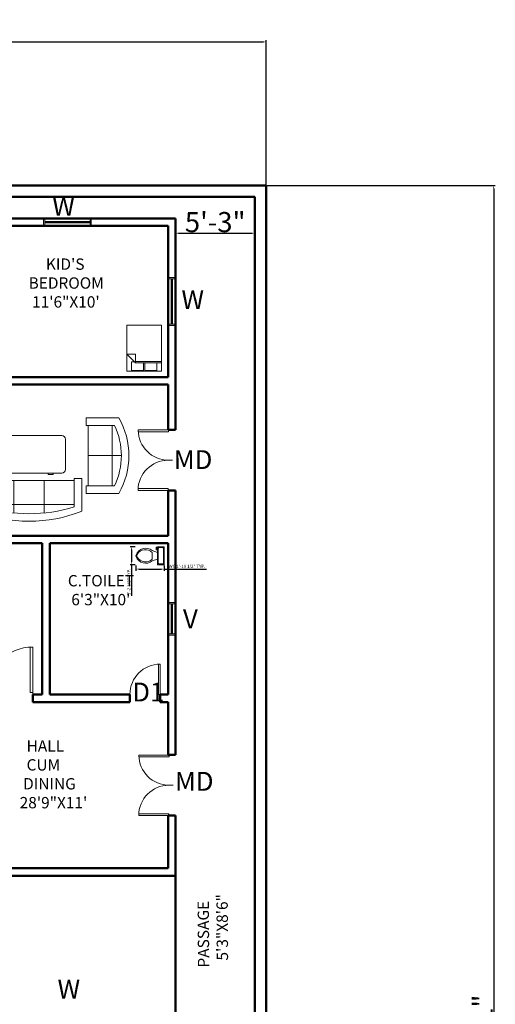
# Model space of a CAD drawing. Units: inches. Extents: x -7040 to -4088, y 6092 to 7645.
# Tile 7 of 11: x -6599 to -6221, y 6864 to 7645. Entities that reach past the tile are written whole.
import ezdxf

# ---------------------------------------------------------------- set-up
doc = ezdxf.new("R2010")
doc.units = ezdxf.units.IN
for name, color, linetype, lineweight in [('A-ANNO-DIMS', 2, 'Continuous', 18), ('A-ANNO-TEXT', 7, 'Continuous', 25), ('A-AREA-IDEN', 3, 'Continuous', 25), ('A-DOOR', 3, 'Continuous', 18), ('A-FLOR-FIXT', 9, 'Continuous', 13), ('A-FURN', 8, 'Continuous', 13), ('A-GLAZ', 4, 'Continuous', 18), ('A-WALL', 7, 'Continuous', 50)]:
    doc.layers.add(name, color=color, linetype=linetype, lineweight=lineweight)
doc.styles.get("Standard").update_dxf_attribs({"font": 'arial.ttf'})
doc.dimstyles.new('ISO-25', dxfattribs={"dimtxt": 2.5, "dimasz": 2.5, "dimexe": 1.25, "dimexo": 0.625, "dimtad": 1, "dimdec": 0, "dimlunit": 3, "dimtxsty": 'Standard', "dimcen": 2.5, "dimadec": 0, "dimazin": 0, "dimtfac": 1, "dimtdec": 0, "dimtmove": 0, "dimatfit": 3, "dimfxl": 1, "dimarcsym": 0})

# ---------------------------------------------------------------- blocks, each defined once
blk = doc.blocks.new('*U8')
for p, q in [((0, 0), (0, -100)), ((750, 0), (750, -100))]:
    blk.add_line(p, q)
blk.add_lwpolyline([(0, 0), (0, 750), (43.75, 750), (43.75, 0)], close=True)
blk.add_arc((0, 0), 750, 0, 90)
blk = doc.blocks.new('Bed - Queen')
for p, q in [((0, -80.00003), (0, 0)), ((0, 0), (59.99999, 0)), ((59.99999, 0), (59.99999, -80.00003)), ((0, -14.4), (44.8, -14.4)), ((44.8, -16.8), (0, -16.8)), ((7.99999, -1.2), (28.79998, -1.2)), ((7.99999, -14.4), (7.99999, -1.2)), ((28.79998, -1.2), (28.79998, -14.4)), ((31.19999, -1.2), (51.99999, -1.2)), ((31.19999, -14.4), (31.19999, -1.2)), ((59.99999, -29.6), (44.8, -14.4)), ((44.8, -14.4), (44.8, -29.6)), ((51.99999, -16.4), (46.79936, -16.4)), ((51.99999, -1.2), (51.99999, -16.4)), ((44.8, -29.6), (59.99999, -29.6)), ((59.99999, -80.00003), (0, -80.00003))]:
    blk.add_line(p, q)
blk = doc.blocks.new('Toilet - top')
for p, q in [((-10, -8.5), (-8, -8.5)), ((-10, -9.5), (-10, -8.5)), ((-7, -9.5), (-10, -9.5)), ((-8, -8.5), (-8, -8)), ((-7, -8), (-7, -9.5)), ((-4, -8), (-6, -14)), ((4, -8), (6, -14)), ((9.5, -6), (9.5, -2)), ((4, -14), (-4, -14))]:
    blk.add_line(p, q)
blk.add_lwpolyline([(10.5, -8), (10.5, 0), (-10.5, 0), (-10.5, -8)], close=True)
for points in [[(-9.5, -2), (-9.5, -6)], [(8.5, -1), (-8.5, -1)], [(-8.5, -7), (8.5, -7)]]:
    blk.add_lwpolyline(points)
for centre, radius, start, end in [((-8.6, -1.9), 0.884, 81.8699, 188.1301), ((-8.6, -6.1), 0.884, 171.8699, 278.1301), ((8.6, -1.9), 0.884, 351.8699, 98.1301), ((8.6, -6.1), 0.884, 261.8699, 8.1301), ((3.5, -21.6), 12.2, 141.4691, 247.9714), ((4.2, -21.8), 11.3, 136.3677, 238.9468), ((-3.5, -21.6), 12.2, 292.0284, 38.5307), ((-4.2, -21.8), 11.3, 301.053, 43.6321), ((0, -27.9), 4, 245.7318, 294.2682), ((0, -29), 4, 254.8605, 285.1395)]:
    blk.add_arc(centre, radius, start, end)
blk = doc.blocks.new('Desk - 30 x 60 in.')
for p, q in [((-26.999995, 0), (26.999995, 0)), ((-29.999995, -27), (-29.999995, -3)), ((29.999995, -3), (29.999995, -27)), ((26.999995, -30), (-26.999995, -30)), ((-20.000005, -30), (-20.000005, -31)), ((-20.000005, -31), (-16.000005, -31)), ((-16.000005, -31), (-16.000005, -30)), ((15.999995, -31), (15.999995, -30)), ((19.999995, -31), (15.999995, -31)), ((19.999995, -30), (19.999995, -31))]:
    blk.add_line(p, q)
for centre, start, end in [((-26.499995, -3.5), 98.1301, 171.8699), ((26.499995, -3.5), 8.130102, 81.8699), ((-26.499995, -26.5), 188.1301, 261.8699), ((26.499995, -26.5), 278.1301, 351.8699)]:
    blk.add_arc(centre, 3.535534, start, end)
blk = doc.blocks.new('Sofa - Roundback 7 ft.')
for p, q in [((-12.00002, -32.4421), (-12.00003, -6.5971)), ((11.99997, -32.4421), (11.99998, -6.5971)), ((-36.000027, -34), (-36.000027, -11.4696)), ((-35.999844, -13.3819), (35.9998, -13.3819)), ((35.99998, -34), (35.99998, -11.4696)), ((-36.000027, -32.4421), (35.99998, -32.4421))]:
    blk.add_line(p, q)
for points in [[(-36.000027, -34), (-42.000027, -34), (-42.000027, -8)], [(41.99998, -8), (41.99998, -34), (35.99998, -34)]]:
    blk.add_lwpolyline(points)
for centre, radius, start, end in [((0, -114.25), 114.25, 68.43141, 111.5686), ((-0.00001, -127.1968), 121.1968, 72.72033, 107.2797)]:
    blk.add_arc(centre, radius, start, end)
blk = doc.blocks.new('Sofa - Roundback Loveseat 5 ft.')
for p, q in [((0, -32.44198), (0, -5.99998)), ((-24, -33.99998), (-24, -11.46958)), ((-23.9998, -13.38178), (23.99986, -13.38178)), ((24.00004, -33.99998), (24.00004, -11.46958)), ((-24, -32.44198), (24.00004, -32.44198))]:
    blk.add_line(p, q)
for points in [[(-24, -33.99998), (-30, -33.99998), (-30, -7.99998)], [(30.00004, -7.99998), (30.00004, -33.99998), (24.00004, -33.99998)]]:
    blk.add_lwpolyline(points)
for centre, radius, start, end in [((0, -60.24998), 60.24998, 60.13715, 119.8628), ((0, -61.38438), 55.38444, 64.32083, 115.6792)]:
    blk.add_arc(centre, radius, start, end)
blk = doc.blocks.new('*D90')
at = {"layer": 'A-ANNO-DIMS', "color": 0, "lineweight": -2, "transparency": 16777216}
for p, q in [((-6475.03, 7487.13), (-6475.03, 7474.72)), ((-6412.03, 7487.13), (-6412.03, 7474.72)), ((-6472.53, 7475.97), (-6414.53, 7475.97))]:
    blk.add_line(p, q, dxfattribs=at)
at = {"layer": 'A-ANNO-DIMS', "color": 0, "transparency": 16777216}
for points in [[(-6472.53, 7476.38), (-6472.53, 7475.55), (-6475.03, 7475.97)], [(-6414.53, 7476.38), (-6414.53, 7475.55), (-6412.03, 7475.97)]]:
    blk.add_solid(points, dxfattribs=at)
at = {"layer": 'Defpoints', "color": 0, "transparency": 16777216}
for p in [(-6475.03, 7487.76), (-6412.03, 7487.76), (-6412.03, 7475.97)]:
    blk.add_point(p, dxfattribs=at)
at = {"layer": 'A-ANNO-DIMS', "color": 0, "transparency": 16777216, "insert": (-6443.53, 7484.77), "char_height": 2.5, "attachment_point": 5}
blk.add_mtext('{\\H6.4x;5\'-3"}', dxfattribs=at)
blk = doc.blocks.new('*D92')
at = {"layer": 'A-ANNO-DIMS', "color": 0, "lineweight": -2, "transparency": 16777216}
for p, q in [((-7003.03, 7514.38), (-7003.03, 7629.1)), ((-7000.53, 7627.85), (-6405.53, 7627.85)), ((-6403.03, 7514.38), (-6403.03, 7629.1))]:
    blk.add_line(p, q, dxfattribs=at)
at = {"layer": 'A-ANNO-DIMS', "color": 0, "transparency": 16777216}
for points in [[(-7000.53, 7628.27), (-7000.53, 7627.43), (-7003.03, 7627.85)], [(-6405.53, 7628.27), (-6405.53, 7627.43), (-6403.03, 7627.85)]]:
    blk.add_solid(points, dxfattribs=at)
at = {"layer": 'Defpoints', "color": 0, "transparency": 16777216}
for p in [(-6403.03, 7627.85), (-7003.03, 7513.76), (-6403.03, 7513.76)]:
    blk.add_point(p, dxfattribs=at)
at = {"layer": 'A-ANNO-DIMS', "color": 0, "transparency": 16777216, "insert": (-6703.03, 7636.64), "char_height": 2.5, "attachment_point": 5}
blk.add_mtext("{\\H6.4x;50'}", dxfattribs=at)
blk = doc.blocks.new('*D93')
at = {"layer": 'A-ANNO-DIMS', "color": 0, "lineweight": -2, "transparency": 16777216}
for p, q in [((-6402.41, 7513.76), (-6220.88, 7513.76)), ((-6222.13, 7511.26), (-6222.13, 6159.26)), ((-6402.41, 6156.76), (-6220.88, 6156.76))]:
    blk.add_line(p, q, dxfattribs=at)
at = {"layer": 'A-ANNO-DIMS', "color": 0, "transparency": 16777216}
for points in [[(-6222.55, 7511.26), (-6221.71, 7511.26), (-6222.13, 7513.76)], [(-6222.55, 6159.26), (-6221.71, 6159.26), (-6222.13, 6156.76)]]:
    blk.add_solid(points, dxfattribs=at)
at = {"layer": 'Defpoints', "color": 0, "transparency": 16777216}
for p in [(-6403.03, 7513.76), (-6403.03, 6156.76), (-6222.13, 6156.76)]:
    blk.add_point(p, dxfattribs=at)
at = {"layer": 'A-ANNO-DIMS', "color": 0, "transparency": 16777216, "insert": (-6230.93, 6835.26), "char_height": 2.5, "attachment_point": 5, "rotation": 90}
blk.add_mtext('{\\H6.4x;113\'-1"}', dxfattribs=at)
blk = doc.blocks.new('WIN-36')
for p, q in [((0, 6), (0, 0)), ((1, 6), (1, 0)), ((1, 3.5), (37, 3.5)), ((1, 3), (37, 3)), ((1, 2.5), (37, 2.5)), ((37, 6), (37, 0)), ((38, 6), (38, 0))]:
    blk.add_line(p, q)
blk = doc.blocks.new('WIN-24')
for p, q in [((0, 6), (0, 0)), ((1, 6), (1, 0)), ((1, 3.5), (25, 3.5)), ((1, 3), (25, 3)), ((1, 2.5), (25, 2.5)), ((25, 6), (25, 0)), ((26, 6), (26, 0))]:
    blk.add_line(p, q)
blk = doc.blocks.new('*D128')
at = {"layer": 'A-ANNO-DIMS', "color": 0, "lineweight": -2, "transparency": 16777216}
for p, q in [((-6506.58, 7212.04), (-6506.58, 7208.03)), ((-6504.08, 7209.28), (-6486.48, 7209.28)), ((-6483.98, 7212.04), (-6483.98, 7208.03)), ((-6483.98, 7209.28), (-6450.33, 7209.28))]:
    blk.add_line(p, q, dxfattribs=at)
at = {"layer": 'A-ANNO-DIMS', "color": 0, "transparency": 16777216}
for points in [[(-6504.08, 7209.7), (-6504.08, 7208.86), (-6506.58, 7209.28)], [(-6486.48, 7209.7), (-6486.48, 7208.86), (-6483.98, 7209.28)]]:
    blk.add_solid(points, dxfattribs=at)
at = {"layer": 'Defpoints', "color": 0, "transparency": 16777216}
for p in [(-6506.58, 7212.67), (-6483.98, 7212.67), (-6483.98, 7209.28)]:
    blk.add_point(p, dxfattribs=at)
at = {"layer": 'A-ANNO-DIMS', "color": 0, "transparency": 16777216, "insert": (-6465.91, 7211.2), "char_height": 2.5, "attachment_point": 5}
blk.add_mtext('WC 1\'-10 1/2" TYP.', dxfattribs=at)
blk = doc.blocks.new('*D129')
at = {"layer": 'A-ANNO-DIMS', "color": 0, "lineweight": -2, "transparency": 16777216}
for p, q in [((-6507.2, 7227.03), (-6511.22, 7227.03)), ((-6509.97, 7224.53), (-6509.97, 7215.17)), ((-6507.2, 7212.67), (-6511.22, 7212.67)), ((-6509.97, 7212.67), (-6509.97, 7188.09))]:
    blk.add_line(p, q, dxfattribs=at)
at = {"layer": 'A-ANNO-DIMS', "color": 0, "transparency": 16777216}
for points in [[(-6510.38, 7224.53), (-6509.55, 7224.53), (-6509.97, 7227.03)], [(-6510.38, 7215.17), (-6509.55, 7215.17), (-6509.97, 7212.67)]]:
    blk.add_solid(points, dxfattribs=at)
at = {"layer": 'Defpoints', "color": 0, "transparency": 16777216}
for p in [(-6506.58, 7227.03), (-6509.97, 7212.67), (-6506.58, 7212.67)]:
    blk.add_point(p, dxfattribs=at)
at = {"layer": 'A-ANNO-DIMS', "color": 0, "transparency": 16777216, "insert": (-6511.89, 7199.13), "char_height": 2.5, "attachment_point": 5, "rotation": 90}
blk.add_mtext('1\'-2 1/2" TYP.', dxfattribs=at)

msp = doc.modelspace()

# ---------------------------------------------------------------- linework, layer by layer
at = {"layer": 'A-WALL'}
for p, q in [((-7003.03, 7513.76), (-6403.03, 7513.76)), ((-6403.03, 7513.76), (-6403.03, 6156.76)), ((-6994.03, 7504.76), (-6412.03, 7504.76)), ((-6412.03, 7504.76), (-6412.03, 6179.76)), ((-6977.03, 7487.76), (-6475.03, 7487.76)), ((-6641.03, 7481.76), (-6481.03, 7481.76)), ((-6481.03, 7481.76), (-6481.03, 7361.76)), ((-6475.03, 7487.76), (-6475.03, 7319.76)), ((-6641.03, 7361.76), (-6481.03, 7361.76)), ((-6845.03, 7355.76), (-6481.03, 7355.76)), ((-6481.03, 7355.76), (-6481.03, 7319.76)), ((-6481.03, 7319.76), (-6475.03, 7319.76)), ((-6481.03, 7271.76), (-6475.03, 7271.76)), ((-6481.03, 7271.76), (-6481.03, 7235.76)), ((-6475.03, 7271.76), (-6475.03, 7061.76)), ((-6845.03, 7235.76), (-6481.03, 7235.76)), ((-6773.03, 7229.76), (-6581.03, 7229.76)), ((-6581.03, 7109.76), (-6581.03, 7229.76)), ((-6575.03, 7109.76), (-6575.03, 7229.76)), ((-6575.03, 7229.76), (-6481.03, 7229.76)), ((-6481.03, 7229.76), (-6481.03, 7109.76)), ((-6588.57, 7109.76), (-6588.57, 7103.76)), ((-6588.57, 7109.76), (-6581.03, 7109.76)), ((-6575.03, 7109.76), (-6511.28, 7109.76)), ((-6511.28, 7109.76), (-6511.28, 7103.76)), ((-6487.28, 7109.76), (-6487.28, 7103.76)), ((-6487.28, 7109.76), (-6481.03, 7109.76)), ((-6588.57, 7103.76), (-6511.28, 7103.76)), ((-6487.28, 7103.76), (-6481.03, 7103.76)), ((-6481.03, 7103.76), (-6481.03, 7061.76)), ((-6481.03, 7061.76), (-6475.03, 7061.76)), ((-6481.03, 7013.76), (-6475.03, 7013.76)), ((-6481.03, 7013.76), (-6481.03, 6971.76)), ((-6475.03, 7013.76), (-6475.03, 6658.26)), ((-6971.03, 6965.76), (-6475.03, 6965.76)), ((-6845.03, 6971.76), (-6481.03, 6971.76))]:
    msp.add_line(p, q, dxfattribs=at)

# ---------------------------------------------------------------- block references
at = {"layer": 'A-DOOR'}
for p, xscale, yscale, zscale, rotation in [((-6480.69, 7319.76), -0.0319999999999999, 0.0319999999999999, 0.0319999999999999, 90), ((-6480.87, 7271.76), 0.0319965751455487, 0.0319965751455487, 0.0319965751455487, 90.00000000000003), ((-6480.16, 7061.66), -0.0319999999999999, 0.0319999999999999, 0.0319999999999999, 90), ((-6480.34, 7013.65), 0.0319965751455487, 0.0319965751455487, 0.0319965751455487, 90.00000000000003)]:
    msp.add_blockref('*U8', p, dxfattribs=dict(at, xscale=xscale, yscale=yscale, zscale=zscale, rotation=rotation))
for p, xscale, yscale, zscale in [((-6588.57, 7111.39), -0.0480000000000005, 0.0480000000000005, 0.0480000000000005), ((-6487.28, 7109.85), -0.0319999981882539, 0.0319999981882539, 0.0319999981882539)]:
    msp.add_blockref('*U8', p, dxfattribs=dict(at, xscale=xscale, yscale=yscale, zscale=zscale))
at = {"layer": 'A-FLOR-FIXT', "xscale": 0.6837915443005316, "yscale": 0.6837915443005316, "zscale": 0.6837915443005316, "rotation": 270}
msp.add_blockref('Toilet - top', (-6483.98, 7219.85), dxfattribs=at)
at = {"layer": 'A-FURN', "xscale": 0.4580400962997241, "yscale": 0.4580400962997241, "zscale": 0.4580400962997241, "rotation": 180}
msp.add_blockref('Bed - Queen', (-6486.3, 7366.43), dxfattribs=at)
at = {"layer": 'A-FURN'}
for name, p, rotation in [('Sofa - Roundback Loveseat 5 ft.', (-6512.11, 7299.37), 270), ('Sofa - Roundback 7 ft.', (-6591.57, 7247.24), 180)]:
    msp.add_blockref(name, p, dxfattribs=dict(at, rotation=rotation))
msp.add_blockref('Desk - 30 x 60 in.', (-6592.41, 7315.38), dxfattribs=at)
at = {"layer": 'A-GLAZ'}
msp.add_blockref('WIN-36', (-6580.03, 7481.76), dxfattribs=at)
for name, p, rotation in [('WIN-36', (-6475.03, 7402.76), 89.99999999999507), ('WIN-24', (-6481.03, 7182.76), 269.9999999999992)]:
    msp.add_blockref(name, p, dxfattribs=dict(at, rotation=rotation))

# ---------------------------------------------------------------- texts
at = {"layer": 'A-ANNO-TEXT', "char_height": 15, "attachment_point": 1}
for s, insert in [('{W}', (-6573.06, 7504.84)), ('{W}', (-6470.39, 7430.73)), ('{MD}', (-6476.46, 7303.7)), ('{V}', (-6469.14, 7177.29)), ('{D1}', (-6509.46, 7119.17)), ('{MD}', (-6475.55, 7048.27)), ('{W}', (-6568.85, 6883.34))]:
    msp.add_mtext_dynamic_manual_height_columns(s, width=701.5203, gutter_width=12.5, heights=[0], dxfattribs=dict(at, insert=insert))
at = {"layer": 'A-AREA-IDEN', "char_height": 9, "attachment_point": 1}
for s, insert in [('{     KID\'S\\PBEDROOM\\P 11\'6"X10\'}', (-6591.84, 7455.91)), ('{  C.TOILET\\P   6\'3"X10\'}', (-6566.15, 7204.57)), ('{  HALL\\P  CUM\\P DINING\\P28\'9"X11\'}', (-6598.95, 7073.36))]:
    msp.add_mtext_dynamic_manual_height_columns(s, width=930.9751, gutter_width=12.5, heights=[0], dxfattribs=dict(at, insert=insert))
at = {"layer": 'A-AREA-IDEN', "insert": (-6457.21, 6881.89), "char_height": 9, "attachment_point": 1, "rotation": 90.30994}
msp.add_mtext_dynamic_manual_height_columns('{    PASSAGE\\P      5\'3"X8\'6"}', width=930.9751, gutter_width=12.5, heights=[0], dxfattribs=at)

# ---------------------------------------------------------------- dimensions: what is measured, and where the dimension line sits
at = {"layer": 'A-ANNO-DIMS'}
for base, p1, p2, text, override, picture, middle in [((-6403.03, 7627.85), (-7003.03, 7513.76), (-6403.03, 7513.76), '{\\H6.4x;<>}', {"dimclrd": 0, "dimclre": 0, "dimclrt": 0}, '*D92', (-6703.03, 7636.64)), ((-6412.03, 7475.97), (-6475.03, 7487.76), (-6412.03, 7487.76), '{\\H6.4x;<>}', {"dimclrd": 0, "dimclre": 0, "dimclrt": 0}, '*D90', (-6443.53, 7484.77)), ((-6483.98, 7209.28), (-6506.58, 7212.67), (-6483.98, 7212.67), 'WC <> TYP.', {"dimdec": 1, "dimrnd": 0, "dimzin": 1, "dimlunit": 4, "dimfrac": 2}, '*D128', (-6465.91, 7211.2))]:
    dim = msp.add_linear_dim(base=base, p1=p1, p2=p2, text=text, dimstyle='ISO-25', override=override, dxfattribs=at)
    dim.commit()
    dim.dimension.update_dxf_attribs({"geometry": picture, "text_midpoint": middle})
for base, p1, p2, angle, text, override, picture, middle in [((-6222.13, 6156.76), (-6403.03, 7513.76), (-6403.03, 6156.76), 90, '{\\H6.4x;<>}', {"dimclrd": 0, "dimclre": 0, "dimclrt": 0}, '*D93', (-6230.93, 6835.26)), ((-6509.97, 7212.67), (-6506.58, 7227.03), (-6506.58, 7212.67), 270, '<> TYP.', {"dimdec": 1, "dimrnd": 0, "dimzin": 1, "dimlunit": 4, "dimfrac": 2}, '*D129', (-6511.89, 7199.13))]:
    dim = msp.add_linear_dim(base=base, p1=p1, p2=p2, angle=angle, text=text, dimstyle='ISO-25', override=override, dxfattribs=at)
    dim.commit()
    dim.dimension.update_dxf_attribs({"geometry": picture, "text_midpoint": middle})

doc.saveas('drawing.dxf')
